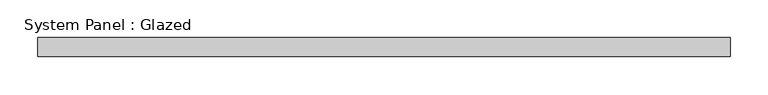
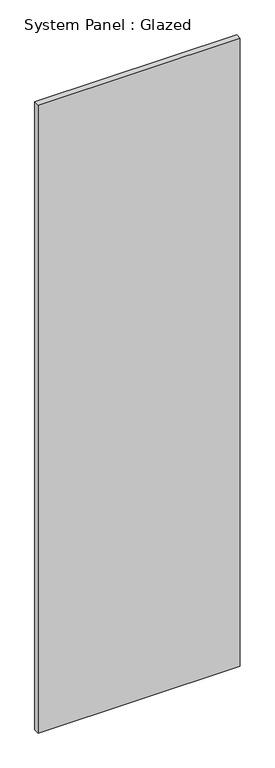
"""IFC4 building model written with IfcOpenShell, lengths in millimetres: plate geometry, System Panel : Glazed."""

from ifc_helpers import new_model, si_unit, origin, origin_with_axes, place, context, project, spatial, polyline, outline, extrude, source, transform, mapped, element, save


def system_panel_glazed_29ba505a(model_context):
    return source(origin(), model_context, "Body", "SweptSolid", [
        extrude(outline(polyline([(457.2, 24.5), (-457.2, 24.5), (-457.2, 49.5), (457.2, 49.5), (457.2, 24.5)])), origin_with_axes(), (0.0, 0.0, 1.0), 3000.0),
    ])


if __name__ == "__main__":
    model = new_model("IFC4")
    model_context = context("Model", 3, world=origin())
    ifc_project = project(units=[si_unit("LENGTHUNIT", "METRE", prefix="MILLI")], contexts=[model_context])
    site = spatial("IfcSite", under=ifc_project)
    building = spatial("IfcBuilding", under=site)
    placement = place(None, origin())
    system_panel_glazed_shape = system_panel_glazed_29ba505a(model_context)
    element("IfcPlate", 1, ObjectType="System Panel : Glazed", at=placement, inside=building, context=model_context, shape_type="MappedRepresentation", body=[
        mapped(system_panel_glazed_shape, transform((0.0, 0.0, 0.0), x_axis=(1.0, 0.0, 0.0), y_axis=(0.0, 1.0, 0.0), z_axis=(0.0, 0.0, 1.0))),
    ])
    save(model, "model.ifc")

# Revit data of these elements
# Type "System Panel : Glazed"
#   Keynote = "H11"
#   Construction Type Id = "GSP4R"
#   Analytic Construction = "1/8 in Pilkington single glazing"
#   Visual Light Transmittance = 0.9
#   Solar Heat Gain Coefficient = 0.86
#   Heat Transfer Coefficient (U) = 6.7069 W/(m²·K)
#   Define Thermal Properties by = 1
# Element 1 (IfcPlate, "System Panel : Glazed")
#   Materials on its faces: "Glass"
# Materials
#   "Glass": class "Glass", colour RGB 0 128 192, transparency 0.9, Description = "Soda Lime Glass", Cost = 0
